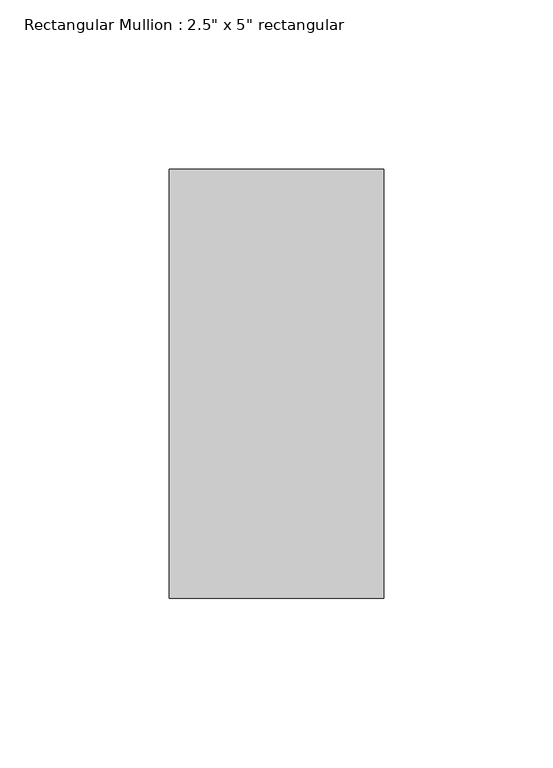
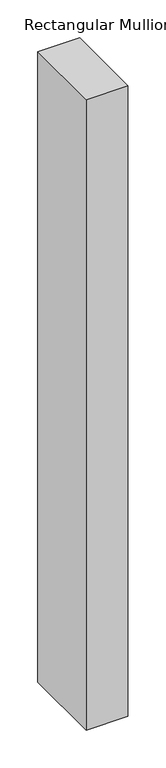
"""IFC4 building model written with IfcOpenShell, lengths in millimetres: member geometry."""

from ifc_helpers import new_model, si_unit, frame, origin, place, context, project, spatial, polyline, outline, extrude, source, transform, mapped, element, save


def member_585633ab(model_context):
    return source(origin(), model_context, "Body", "SweptSolid", [
        extrude(outline(polyline([(0.0, 63.5), (0.0, -63.5), (-63.5, -63.5), (-63.5, 63.5), (0.0, 63.5)])), frame((0.0, 0.0, -1014.4047405), z_axis=(0.0, 0.0, 1.0), x_axis=(1.0, 0.0, 0.0)), (0.0, 0.0, 1.0), 1014.4047405),
    ])


if __name__ == "__main__":
    model = new_model("IFC4")
    model_context = context("Model", 3, world=origin())
    ifc_project = project(units=[si_unit("LENGTHUNIT", "METRE", prefix="MILLI")], contexts=[model_context])
    site = spatial("IfcSite", under=ifc_project)
    building = spatial("IfcBuilding", under=site)
    placement = place(None, origin())
    member_shape = member_585633ab(model_context)
    element("IfcMember", 1, ObjectType="Rectangular Mullion : 2.5\" x 5\" rectangular", at=placement, inside=building, context=model_context, shape_type="MappedRepresentation", body=[
        mapped(member_shape, transform((0.0, 0.0, 0.0), x_axis=(1.0, 0.0, 0.0), y_axis=(0.0, 1.0, 0.0), z_axis=(0.0, 0.0, 1.0))),
    ])
    save(model, "model.ifc")

# Revit data of these elements
# Type "Rectangular Mullion : 2.5\" x 5\" rectangular"
#   built-in parameter 1007304 = 0.416667 (stored number, unit not read)
#   built-in parameter 1007301 = 0.104167 (stored number, unit not read)
#   built-in parameter 1007300 = 0.104167 (stored number, unit not read)
